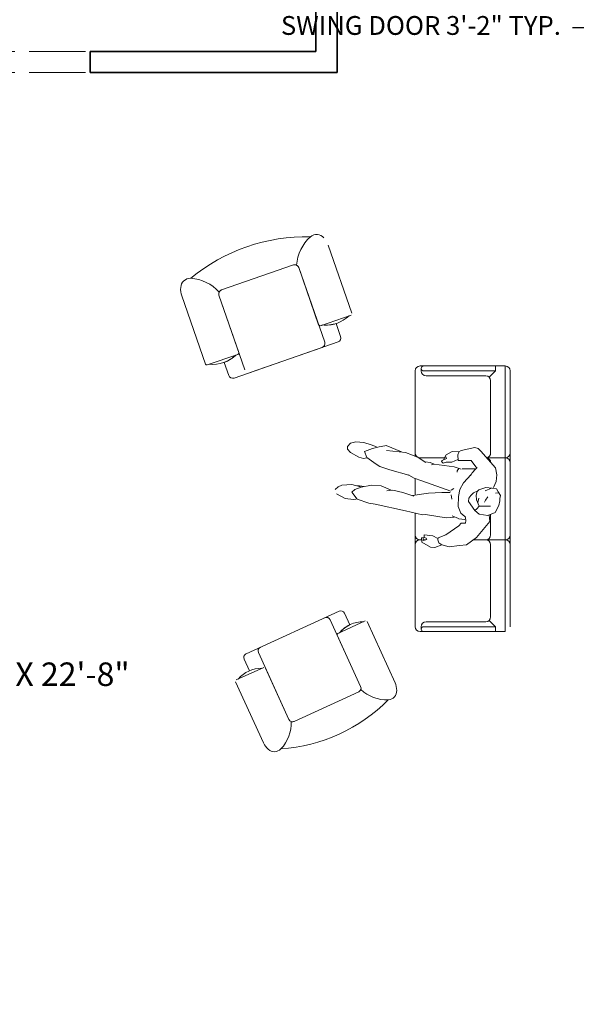
# Model space of a CAD drawing. Units: inches. Extents: x -638 to 186, y -762 to 59.
# Tile 14 of 31: x -287 to -168, y -413 to -203. Entities that reach past the tile are written whole.
import ezdxf

# ---------------------------------------------------------------- set-up
doc = ezdxf.new("R2010")
doc.units = ezdxf.units.IN
doc.linetypes.add('ACAD_ISO02W100', pattern=[15, 12, -3])
for name, color, linetype, lineweight in [('A-ANNO-DIMS', 2, 'Continuous', 18), ('A-AREA-IDEN', 1, 'Continuous', 18), ('A-ENTG-PEPL', 251, 'Continuous', 9), ('A-WALL-OVHD', 1, 'ACAD_ISO02W100', 18), ('furn', 8, 'Continuous', 13), ('wall', 7, 'Continuous', 35)]:
    doc.layers.add(name, color=color, linetype=linetype, lineweight=lineweight)
doc.styles.get("Standard").update_dxf_attribs({"font": 'arial.ttf'})
doc.dimstyles.new('ISO-25', dxfattribs={"dimtxt": 4, "dimasz": 4, "dimexe": 1.25, "dimexo": 0.625, "dimtad": 0, "dimlunit": 4, "dimtxsty": 'Standard', "dimcen": 2.5, "dimclrt": 256, "dimadec": 0, "dimazin": 0, "dimtfac": 1, "dimtmove": 0, "dimatfit": 3, "dimfxl": 1, "dimfxlon": 1, "dimarcsym": 0})

# ---------------------------------------------------------------- blocks, each defined once
blk = doc.blocks.new('*D23')
at = {"layer": 'A-ANNO-DIMS', "color": 0, "lineweight": -2, "transparency": 16777216}
for p, q in [((-165.01, -205.03), (-169.01, -205.03)), ((-165.01, -204.03), (-165.01, -206.28)), ((-131.22, -205.03), (-161.01, -205.03)), ((-127.22, -204.03), (-127.22, -206.28))]:
    blk.add_line(p, q, dxfattribs=at)
at = {"layer": 'A-ANNO-DIMS', "color": 0, "lineweight": 30, "transparency": 16777216}
for points in [[(-161.01, -204.37), (-161.01, -205.7), (-165.01, -205.03)], [(-131.22, -204.37), (-131.22, -205.7), (-127.22, -205.03)]]:
    blk.add_solid(points, dxfattribs=at)
at = {"layer": 'Defpoints', "color": 0, "lineweight": 30, "transparency": 16777216}
for p in [(-165.01, -199.36), (-127.22, -199.36), (-165.01, -205.03)]:
    blk.add_point(p, dxfattribs=at)
at = {"layer": 'A-ANNO-DIMS', "transparency": 16777216, "insert": (-201.22, -205.03), "char_height": 4, "attachment_point": 5}
blk.add_mtext('SWING DOOR 3\'-2" TYP.', dxfattribs=at)
blk = doc.blocks.new('*D37')
at = {"layer": 'A-ANNO-DIMS', "color": 0, "lineweight": -2, "transparency": 16777216}
for p, q in [((182.66, -232.53), (184.91, -232.53)), ((183.66, -236.53), (183.66, -250.51)), ((183.66, -276.53), (183.66, -262.56)), ((182.66, -280.53), (184.91, -280.53))]:
    blk.add_line(p, q, dxfattribs=at)
at = {"layer": 'A-ANNO-DIMS', "color": 0, "lineweight": 30, "transparency": 16777216}
for points in [[(183, -236.53), (184.33, -236.53), (183.66, -232.53)], [(183, -276.53), (184.33, -276.53), (183.66, -280.53)]]:
    blk.add_solid(points, dxfattribs=at)
at = {"layer": 'Defpoints', "color": 0, "lineweight": 30, "transparency": 16777216}
for p in [(-404.53, -232.53), (-404.53, -280.53), (183.66, -280.53)]:
    blk.add_point(p, dxfattribs=at)
at = {"layer": 'A-ANNO-DIMS', "transparency": 16777216, "insert": (183.66, -256.53), "char_height": 4, "attachment_point": 5, "rotation": 90}
blk.add_mtext('4\'-0"', dxfattribs=at)
blk = doc.blocks.new('*D38')
at = {"layer": 'A-ANNO-DIMS', "color": 0, "lineweight": -2, "transparency": 16777216}
for p, q in [((182.66, -280.53), (184.91, -280.53)), ((183.66, -284.53), (183.66, -371.73)), ((183.66, -473.53), (183.66, -386.34)), ((182.66, -477.53), (184.91, -477.53))]:
    blk.add_line(p, q, dxfattribs=at)
at = {"layer": 'A-ANNO-DIMS', "color": 0, "lineweight": 30, "transparency": 16777216}
for points in [[(183, -284.53), (184.33, -284.53), (183.66, -280.53)], [(183, -473.53), (184.33, -473.53), (183.66, -477.53)]]:
    blk.add_solid(points, dxfattribs=at)
at = {"layer": 'Defpoints', "color": 0, "lineweight": 30, "transparency": 16777216}
for p in [(-404.53, -280.53), (-404.53, -477.53), (183.66, -477.53)]:
    blk.add_point(p, dxfattribs=at)
at = {"layer": 'A-ANNO-DIMS', "transparency": 16777216, "insert": (183.66, -379.03), "char_height": 4, "attachment_point": 5, "rotation": 90}
blk.add_mtext('16\'-5"', dxfattribs=at)
blk = doc.blocks.new('*D39')
at = {"layer": 'A-ANNO-DIMS', "color": 0, "lineweight": -2, "transparency": 16777216}
for p, q in [((-344.53, -751.58), (-344.53, -753.83)), ((-340.53, -752.58), (-313.98, -752.58)), ((-275.53, -752.58), (-302.07, -752.58)), ((-271.53, -751.58), (-271.53, -753.83))]:
    blk.add_line(p, q, dxfattribs=at)
at = {"layer": 'A-ANNO-DIMS', "color": 0, "lineweight": 30, "transparency": 16777216}
for points in [[(-340.53, -751.92), (-340.53, -753.25), (-344.53, -752.58)], [(-275.53, -751.92), (-275.53, -753.25), (-271.53, -752.58)]]:
    blk.add_solid(points, dxfattribs=at)
at = {"layer": 'Defpoints', "color": 0, "lineweight": 30, "transparency": 16777216}
for p in [(-344.53, -214.53), (-271.53, -214.53), (-271.53, -752.58)]:
    blk.add_point(p, dxfattribs=at)
at = {"layer": 'A-ANNO-DIMS', "transparency": 16777216, "insert": (-308.03, -752.58), "char_height": 4, "attachment_point": 5}
blk.add_mtext('6\'-1"', dxfattribs=at)

msp = doc.modelspace()

# ---------------------------------------------------------------- linework, layer by layer
at = {"layer": 'A-ENTG-PEPL'}
for p, q in [((-216.835, -293.995, -103.961), (-216.211, -293.311, -103.961)), ((-216.815, -294.538, -103.961), (-216.835, -293.995, -103.961)), ((-216.177, -295.242, -103.961), (-216.815, -294.538, -103.961)), ((-216.211, -293.311, -103.961), (-215.063, -292.962, -103.961)), ((-215.063, -292.962, -103.961), (-213.387, -293.116, -103.961)), ((-213.387, -293.116, -103.961), (-211.817, -293.608, -103.961)), ((-213.188, -295.08, -103.961), (-211.493, -294.43, -103.961)), ((-211.817, -293.608, -103.961), (-210.649, -294.059, -103.961)), ((-211.493, -294.43, -103.961), (-210.106, -294.039, -103.961)), ((-210.106, -294.039, -103.961), (-208.904, -293.867, -103.961)), ((-208.904, -293.867, -103.961), (-208.573, -293.753, -103.961)), ((-208.573, -293.753, -103.961), (-205.378, -295.108, -103.961)), ((-208.52, -294.842, -103.961), (-204.514, -295.28, -103.961)), ((-195.875, -295.771), (-194.564, -295.027)), ((-194.564, -295.027), (-193.121, -295.142)), ((-193.121, -295.142), (-192.669, -294.855)), ((-192.669, -294.855), (-189.735, -294.232)), ((-189.735, -294.232), (-189.03, -294.413)), ((-189.03, -294.413), (-188.458, -294.991)), ((-188.458, -294.991), (-185.351, -298.556, -103.961)), ((-214.414, -296.274, -103.961), (-216.177, -295.242, -103.961)), ((-213.436, -296.52, -103.961), (-214.414, -296.274, -103.961)), ((-212.735, -296.388, -103.961), (-213.436, -296.52, -103.961)), ((-212.688, -296.316, -103.961), (-213.188, -295.08, -103.961)), ((-210.712, -297.729, -103.961), (-212.688, -296.316, -103.961)), ((-204.514, -295.28, -103.961), (-202.973, -295.856, -103.961)), ((-202.973, -295.856, -103.961), (-201.815, -296.356, -103.961)), ((-201.815, -296.356, -103.961), (-200.175, -297.401, -103.961)), ((-196.67, -296.982), (-196.806, -297.191)), ((-196.67, -296.982), (-195.765, -296.518)), ((-196.32, -296.676), (-195.875, -295.771)), ((-195.765, -296.518), (-195.896, -296.159)), ((-193.355, -296.756), (-194.665, -297.298)), ((-193.127, -295.196), (-193.37, -295.735)), ((-193.37, -295.735), (-193.317, -296.948)), ((-193.317, -296.948), (-190.55, -296.991)), ((-190.55, -296.991), (-189.32, -298.565, -103.961)), ((-209.917, -298.247, -103.961), (-210.712, -297.729, -103.961)), ((-207.845, -298.929, -103.961), (-209.917, -298.247, -103.961)), ((-203.782, -300.115, -103.961), (-207.845, -298.929, -103.961)), ((-200.331, -297.281, -103.961), (-199.269, -297.364, -103.961)), ((-199.269, -297.364, -103.961), (-198.397, -297.755, -103.961)), ((-198.931, -297.919, -103.961), (-198.39, -297.718, -103.961)), ((-198.39, -297.718, -103.961), (-194.161, -298.329, -103.961)), ((-196.513, -297.53), (-196.806, -297.191)), ((-195.867, -297.33), (-196.513, -297.53)), ((-194.665, -297.298), (-195.867, -297.33)), ((-194.161, -298.329, -103.961), (-192.64, -298.812, -103.961)), ((-193.188, -298.664, -103.961), (-193.508, -299.125, -103.961)), ((-193.508, -299.125, -103.961), (-193.486, -299.452, -103.961)), ((-192.45, -298.76, -103.961), (-191.409, -298.749, -103.961)), ((-191.409, -298.749, -103.961), (-189.755, -298.757, -103.961)), ((-189.629, -298.834, -103.961), (-190.319, -299.594, -103.961)), ((-189.226, -298.484, -103.961), (-189.629, -298.834, -103.961)), ((-185.351, -298.556, -103.961), (-185.049, -299.992, -103.961)), ((-203.782, -300.115, -103.961), (-203.821, -299.978, -103.961)), ((-202.685, -300.726, -103.961), (-203.782, -300.115, -103.961)), ((-200.998, -301.28, -103.961), (-202.685, -300.726, -103.961)), ((-194.89, -303.475, -103.961), (-200.998, -301.28, -103.961)), ((-190.524, -299.913, -103.961), (-192.137, -301.697, -103.961)), ((-190.319, -299.594, -103.961), (-190.679, -300.242, -103.961)), ((-185.049, -299.992, -103.961), (-185.211, -301.458, -103.961)), ((-219.423, -303.098, -103.961), (-218.814, -302.584, -103.961)), ((-218.814, -302.584, -103.961), (-218.02, -302.204, -103.961)), ((-218.02, -302.204, -103.961), (-215.922, -302.044, -103.961)), ((-215.922, -302.044, -103.961), (-214.027, -302.563, -103.961)), ((-215.893, -303.705, -103.961), (-215.286, -303.107, -103.961)), ((-215.286, -303.107, -103.961), (-213.932, -302.62, -103.961)), ((-214.668, -302.298, -103.961), (-213.373, -302.519, -103.961)), ((-213.932, -302.62, -103.961), (-211.693, -302.205, -103.961)), ((-211.693, -302.205, -103.961), (-209.641, -302.372, -103.961)), ((-209.641, -302.372, -103.961), (-207.54, -303.263, -103.961)), ((-208.489, -303.396, -103.961), (-207.152, -303.296, -103.961)), ((-207.152, -303.296, -103.961), (-205.035, -303.762, -103.961)), ((-194.786, -303.274, -103.961), (-194.204, -302.912, -103.961)), ((-192.965, -303.149, -103.961), (-193.25, -304.581, -103.961)), ((-192.137, -301.697, -103.961), (-192.965, -303.149, -103.961)), ((-189.126, -303.386, -103.961), (-190.044, -303.82, -103.961)), ((-188.931, -303.195, -103.961), (-189.227, -303.585, -103.961)), ((-187.394, -302.692, -103.961), (-188.931, -303.195, -103.961)), ((-187.557, -303.377, -103.961), (-186.242, -302.844, -103.961)), ((-186.071, -302.814, -103.961), (-187.394, -302.692, -103.961)), ((-185.15, -302.959, -103.961), (-186.071, -302.814, -103.961)), ((-185.211, -301.458, -103.961), (-185.814, -302.686, -103.961)), ((-184.801, -303.657, -103.961), (-185.15, -302.959, -103.961)), ((-217.289, -305.044, -103.961), (-219.156, -304.044, -103.961)), ((-215.536, -305.265, -103.961), (-217.289, -305.044, -103.961)), ((-214.78, -305.19, -103.961), (-215.893, -303.705, -103.961)), ((-215.07, -305.178, -103.961), (-215.536, -305.265, -103.961)), ((-212.314, -306.034, -103.961), (-214.78, -305.19, -103.961)), ((-205.035, -303.762, -103.961), (-202.744, -304.521, -103.961)), ((-202.994, -304.404, -103.961), (-199.629, -303.94, -103.961)), ((-199.629, -303.94, -103.961), (-196.765, -303.74, -103.961)), ((-196.765, -303.74, -103.961), (-194.968, -303.738, -103.961)), ((-194.631, -305.204, -103.961), (-194.805, -304.271, -103.961)), ((-193.25, -304.581, -103.961), (-193.275, -306.77, -103.961)), ((-190.993, -304.979, -103.961), (-191.08, -305.71, -103.961)), ((-190.606, -304.388, -103.961), (-190.993, -304.979, -103.961)), ((-190.044, -303.82, -103.961), (-190.606, -304.388, -103.961)), ((-189.227, -303.585, -103.961), (-189.468, -304.345, -103.961)), ((-189.468, -304.345, -103.961), (-189.398, -305.347, -103.961)), ((-189.398, -305.347, -103.961), (-188.815, -306.67, -103.961)), ((-188.92, -304.942, -103.961), (-189.136, -305.883, -103.961)), ((-187.478, -305.37, -103.961), (-187.725, -305.823, -103.961)), ((-186.993, -304.697, -103.961), (-187.478, -305.37, -103.961)), ((-184.78, -303.802, -103.961), (-185.339, -303.91, -103.961)), ((-184.317, -304.383, -103.961), (-184.801, -303.657, -103.961)), ((-184.454, -305.044, -103.961), (-184.317, -304.383, -103.961)), ((-184.412, -305.57, -103.961), (-184.454, -305.044, -103.961)), ((-210.974, -306.263, -103.961), (-212.314, -306.034, -103.961)), ((-204.51, -307.639, -103.961), (-210.974, -306.263, -103.961)), ((-193.275, -306.77, -103.961), (-192.748, -308.184, -103.961)), ((-191.08, -305.71, -103.961), (-189.719, -307.557, -103.961)), ((-189.335, -307.229, -103.961), (-189.719, -307.557, -103.961)), ((-189.719, -307.557, -103.961), (-188.833, -308.373, -103.961)), ((-188.815, -306.67, -103.961), (-189.335, -307.229, -103.961)), ((-188.789, -306.694, -103.961), (-186.434, -306.685, -103.961)), ((-185.439, -308.022, -103.961), (-184.66, -306.56, -103.961)), ((-184.66, -306.56, -103.961), (-184.412, -305.57, -103.961)), ((-200.893, -308.488, -103.961), (-204.51, -307.639, -103.961)), ((-200.254, -308.435, -103.961), (-200.893, -308.488, -103.961)), ((-195.813, -309.14, -103.961), (-200.254, -308.435, -103.961)), ((-194.151, -308.971, -103.961), (-195.813, -309.14, -103.961)), ((-193.238, -309.293, -103.961), (-194.562, -308.721, -103.961)), ((-191.848, -309.531, -103.961), (-193.162, -309.359, -103.961)), ((-192.748, -308.184, -103.961), (-191.901, -308.892, -103.961)), ((-191.787, -308.773, -103.961), (-191.663, -309.696, -103.961)), ((-188.833, -308.373, -103.961), (-186.964, -308.655, -103.961)), ((-186.964, -308.655, -103.961), (-185.439, -308.022, -103.961)), ((-186.593, -309.949, -103.961), (-186.67, -308.534, -103.961)), ((-193.152, -310.851, -103.961), (-195.932, -312.79, -103.961)), ((-192.639, -310.301, -103.961), (-193.152, -310.851, -103.961)), ((-191.71, -310.275, -103.961), (-192.639, -310.301, -103.961)), ((-191.663, -309.696, -103.961), (-191.71, -310.275, -103.961)), ((-189.365, -313.299, -103.961), (-186.593, -309.949, -103.961)), ((-199.973, -313.761, -103.961), (-200.745, -313.967, -103.961)), ((-200.503, -312.769, -103.961), (-200.56, -313.334, -103.961)), ((-200.56, -313.334, -103.961), (-200.123, -313.481, -103.961)), ((-198.655, -312.994, -103.961), (-200.503, -312.769, -103.961)), ((-200.123, -313.481, -103.961), (-199.973, -313.761, -103.961)), ((-197.618, -313.546, -103.961), (-198.655, -312.994, -103.961)), ((-197.647, -313.801, -103.961), (-197.579, -313.371, -103.961)), ((-197.41, -314.432, -103.961), (-197.647, -313.801, -103.961)), ((-195.932, -312.79, -103.961), (-197.579, -313.371, -103.961)), ((-191.503, -314.852, -103.961), (-189.365, -313.299, -103.961)), ((-199.185, -315.357, -103.961), (-198.267, -315.446, -103.961)), ((-198.267, -315.446, -103.961), (-196.79, -314.918, -103.961)), ((-196.79, -314.918, -103.961), (-197.41, -314.432, -103.961)), ((-196.79, -314.918, -103.961), (-195.242, -315.29, -103.961)), ((-195.242, -315.29, -103.961), (-193.029, -315.062, -103.961)), ((-193.029, -315.062, -103.961), (-191.503, -314.852, -103.961))]:
    msp.add_line(p, q, dxfattribs=at)
at = {"layer": 'A-ENTG-PEPL', "elevation": -103.961}
msp.add_lwpolyline([(-200.745, -313.967), (-200.703, -313.293), (-201.105, -313.383), (-201.046, -314.329), (-199.185, -315.357)], dxfattribs=at)
at = {"layer": 'A-WALL-OVHD'}
for p, q in [((-344.526, -210.033), (-271.526, -210.033)), ((-344.526, -214.533), (-271.526, -214.533))]:
    msp.add_line(p, q, dxfattribs=at)
at = {"layer": 'furn'}
for p, q in [((-215.879, -265.669), (-220.912, -251.167)), ((-243.612, -260.703), (-228.325, -255.398)), ((-228.325, -255.398), (-243.612, -260.703)), ((-228.325, -255.398), (-243.612, -260.703)), ((-227.181, -255.952), (-222.956, -268.125)), ((-227.181, -255.952), (-222.956, -268.125)), ((-221.679, -271.806), (-227.181, -255.952)), ((-247.019, -276.476), (-252.052, -261.974)), ((-239.942, -274.02), (-244.166, -261.847)), ((-244.166, -261.847), (-238.665, -277.7)), ((-244.166, -261.847), (-239.942, -274.02)), ((-222.575, -268.31), (-216.064, -266.051)), ((-222.575, -268.31), (-222.15, -268.163)), ((-219.242, -267.861), (-218.282, -270.627)), ((-218.836, -271.771), (-240.918, -279.434)), ((-237.521, -278.255), (-222.234, -272.95)), ((-240.127, -274.401), (-246.638, -276.661)), ((-242.062, -278.879), (-243.022, -276.114)), ((-240.551, -274.549), (-240.127, -274.401)), ((-202.44, -277.914), (-202.44, -296.086)), ((-200.642, -276.878), (-201.405, -276.878)), ((-201.16, -277.396), (-201.16, -277.914)), ((-200.642, -276.878), (-183.283, -276.878)), ((-185.354, -277.914), (-200.642, -277.914)), ((-186.693, -279.253), (-185.354, -277.914)), ((-185.354, -277.914), (-185.354, -276.878)), ((-182.247, -277.914), (-182.247, -332.28)), ((-200.124, -278.949), (-187.425, -278.949)), ((-186.389, -279.985), (-186.389, -295.345)), ((-196.175, -296.381), (-201.405, -296.381)), ((-183.283, -296.381), (-187.247, -296.381)), ((-202.44, -300.807), (-202.44, -304.328)), ((-202.44, -308.125), (-202.44, -332.28)), ((-186.389, -308.417), (-186.389, -312.777)), ((-201.078, -313.813), (-201.405, -313.813)), ((-200.168, -313.813), (-200.735, -313.813)), ((-183.283, -313.813), (-190.072, -313.813)), ((-186.389, -314.848), (-186.389, -330.209)), ((-218.594, -328.993), (-238.404, -338.051)), ((-216.35, -331.887), (-217.484, -329.406)), ((-220.532, -330.8), (-214.029, -345.022)), ((-218.884, -333.731), (-213.043, -331.06)), ((-212.673, -331.198), (-206.724, -344.209)), ((-201.16, -332.797), (-201.16, -332.28)), ((-185.354, -332.28), (-200.642, -332.28)), ((-187.425, -331.244), (-200.124, -331.244)), ((-186.693, -330.941), (-185.354, -332.28)), ((-185.354, -332.28), (-185.354, -333.315)), ((-214.029, -345.022), (-219.022, -334.101)), ((-214.029, -345.022), (-219.022, -334.101)), ((-218.884, -333.731), (-218.503, -333.557)), ((-200.642, -333.315), (-201.405, -333.315)), ((-183.283, -333.315), (-200.642, -333.315)), ((-229.267, -351.99), (-235.77, -337.767)), ((-234.63, -340.931), (-240.472, -343.602)), ((-238.818, -339.161), (-237.683, -341.642)), ((-229.267, -351.99), (-234.26, -341.069)), ((-234.26, -341.069), (-229.267, -351.99)), ((-240.61, -343.972), (-234.661, -356.983)), ((-214.442, -346.132), (-228.157, -352.403)), ((-214.442, -346.132), (-228.157, -352.403)), ((-228.157, -352.403), (-214.442, -346.132))]:
    msp.add_line(p, q, dxfattribs=at)
msp.add_lwpolyline([(-183.283, -276.878), (-183.283, -333.315)], dxfattribs=at)
for centre, radius, start, end in [((-223.381, -251.032), 2.098, 42.15096, 129.53897), ((-225.567, -288.022), 38.617, 88.73747, 129.53993), ((-218.732, -256.037), 8.926, 132.10071, 176.15197), ((-218.732, -256.037), 8.926, 132.10071, 176.15197), ((-228.03, -256.247), 0.899, 64.1387, 109.1387), ((-228.03, -256.247), 0.899, 19.1387, 109.1387), ((-228.03, -256.247), 0.899, 64.1387, 109.1387), ((-228.03, -256.247), 0.899, 19.1387, 64.1387), ((-228.03, -256.247), 0.899, 19.1387, 64.1387), ((-250.198, -260.338), 2.098, 88.73843, 176.12644), ((-250.747, -267.148), 8.926, 42.12543, 86.17668), ((-250.747, -267.148), 8.926, 42.12543, 86.17668), ((-247.806, -260.5), 4.495, 176.12644, 199.1387), ((-243.317, -261.552), 0.899, 109.1387, 199.1387), ((-243.317, -261.552), 0.899, 154.1387, 199.1387), ((-243.317, -261.552), 0.899, 154.1387, 199.1387), ((-243.317, -261.552), 0.899, 109.1387, 154.1387), ((-243.317, -261.552), 0.899, 109.1387, 154.1387), ((-221.406, -261.166), 7.036, 263.93143, 314.34596), ((-222.673, -268.027), 0.3, 199.1387, 289.1387), ((-222.673, -268.027), 0.3, 199.1387, 289.1387), ((-221.406, -261.166), 7.036, 263.93143, 287.91851), ((-222.528, -272.1), 0.899, 289.1387, 19.1387), ((-219.131, -270.921), 0.899, 289.1387, 19.1387), ((-240.225, -274.118), 0.3, 289.1387, 19.1387), ((-240.225, -274.118), 0.3, 289.1387, 19.1387), ((-245.469, -269.517), 7.036, 263.93143, 314.34596), ((-245.469, -269.517), 7.036, 290.35889, 314.34596), ((-246.736, -276.378), 0.3, 199.1387, 289.1387), ((-201.405, -277.914), 1.036, 90, 180), ((-200.642, -277.396), 0.518, 90, 270), ((-200.124, -277.914), 1.036, 180, 270), ((-183.283, -277.914), 1.036, 0, 90), ((-241.213, -278.584), 0.899, 199.1387, 289.1387), ((-187.425, -279.985), 1.036, 0, 90), ((-201.405, -295.345), 1.036, 180, 270), ((-201.405, -297.417), 1.036, 90, 106.92048), ((-187.425, -295.345), 1.036, 279.2298, 0), ((-187.425, -297.417), 1.036, 0, 79.2183), ((-183.283, -295.345), 1.036, 270, 0), ((-183.283, -297.417), 1.036, 0, 90), ((-201.405, -312.777), 1.036, 180, 270), ((-201.405, -314.848), 1.036, 90, 180), ((-187.425, -312.777), 1.036, 270, 0), ((-187.425, -314.848), 1.036, 0, 90), ((-183.283, -312.777), 1.036, 270, 0), ((-183.283, -314.848), 1.036, 0, 90), ((-221.294, -331.148), 0.838, 24.57225, 114.57225), ((-218.246, -329.755), 0.838, 24.57225, 114.57225), ((-187.425, -330.209), 1.036, 270, 0), ((-213.497, -337.791), 6.557, 89.36499, 139.77951), ((-213.497, -337.791), 6.557, 115.79244, 139.77951), ((-201.405, -332.28), 1.036, 180, 270), ((-200.124, -332.28), 1.036, 90, 180), ((-200.642, -332.797), 0.518, 90, 270), ((-218.768, -333.985), 0.279, 114.57225, 204.57225), ((-218.768, -333.985), 0.279, 114.57225, 204.57225), ((-235.008, -337.419), 0.838, 114.57225, 204.57225), ((-238.056, -338.813), 0.838, 114.57225, 204.57225), ((-235.084, -347.662), 6.557, 89.36499, 139.77951), ((-214.79, -345.371), 0.838, 294.57225, 24.57225), ((-214.79, -345.371), 0.838, 339.57225, 24.57225), ((-214.79, -345.371), 0.838, 339.57225, 24.57225), ((-210.533, -345.951), 4.189, 1.55999, 24.57225), ((-214.79, -345.371), 0.838, 294.57225, 339.57225), ((-214.79, -345.371), 0.838, 294.57225, 339.57225), ((-208.392, -339.524), 8.319, 227.55898, 271.61023), ((-208.392, -339.524), 8.319, 227.55898, 271.61023), ((-208.3, -345.89), 1.955, 274.17198, 1.55999), ((-233.594, -322.38), 35.989, 274.17102, 314.97348), ((-237.113, -352.657), 8.319, 317.53427, 1.58552), ((-237.113, -352.657), 8.319, 317.53427, 1.58552), ((-228.505, -351.641), 0.838, 204.57225, 294.57225), ((-228.505, -351.641), 0.838, 204.57225, 249.57225), ((-228.505, -351.641), 0.838, 204.57225, 249.57225), ((-228.505, -351.641), 0.838, 249.57225, 294.57225), ((-228.505, -351.641), 0.838, 249.57225, 294.57225), ((-230.851, -355.241), 4.189, 204.57225, 227.58451), ((-232.358, -356.89), 1.955, 227.58451, 314.97252)]:
    msp.add_arc(centre, radius, start, end, dxfattribs=at)
at = {"layer": 'wall'}
for p, q in [((-223.526, -210.033), (-223.526, -97.533)), ((-219.026, -214.533), (-219.026, -153.025)), ((-271.526, -214.533), (-271.526, -210.033)), ((-271.526, -210.033), (-223.526, -210.033)), ((-271.526, -214.533), (-223.526, -214.533)), ((-223.526, -214.533), (-219.026, -214.533))]:
    msp.add_line(p, q, dxfattribs=at)

# ---------------------------------------------------------------- texts
at = {"layer": 'A-AREA-IDEN', "insert": (-315.786, -329.852), "char_height": 5, "attachment_point": 1}
msp.add_mtext_dynamic_manual_height_columns('\\A1;LIVING\\P19\'-11 {\\H0.7x;\\S1/2;}" X 22\'-8"', width=96.10133, gutter_width=12.5, heights=[0], dxfattribs=at)

# ---------------------------------------------------------------- dimensions: what is measured, and where the dimension line sits
at = {"layer": 'A-ANNO-DIMS'}
dim = msp.add_linear_dim(base=(-165.015, -205.032), p1=(-127.219, -199.363), p2=(-165.015, -199.363), angle=180, text='SWING DOOR <> TYP.', dimstyle='ISO-25', override={"dimdec": 1, "dimlfac": 1, "dimrnd": 0, "dimzin": 1, "dimdsep": 46, "dimlunit": 4, "dimfrac": 2}, dxfattribs=at)
dim.commit()
dim.dimension.update_dxf_attribs({"geometry": '*D23', "text_midpoint": (-201.224, -205.032)})
dim = msp.add_linear_dim(base=(-271.526, -752.583), p1=(-344.526, -214.533), p2=(-271.526, -214.533), dimstyle='ISO-25', override={"dimdec": 1, "dimlfac": 1, "dimrnd": 0, "dimzin": 1, "dimdsep": 46, "dimlunit": 4, "dimfrac": 2}, dxfattribs=at)
dim.commit()
dim.dimension.update_dxf_attribs({"geometry": '*D39', "text_midpoint": (-308.026, -752.583)})
for base, p1, p2, picture, middle in [((183.663, -280.533), (-404.526, -232.533), (-404.526, -280.533), '*D37', (183.663, -256.533)), ((183.663, -477.533), (-404.526, -280.533), (-404.526, -477.533), '*D38', (183.663, -379.033))]:
    dim = msp.add_linear_dim(base=base, p1=p1, p2=p2, angle=90, dimstyle='ISO-25', override={"dimdec": 1, "dimlfac": 1, "dimrnd": 0, "dimzin": 1, "dimdsep": 46, "dimlunit": 4, "dimfrac": 2}, dxfattribs=at)
    dim.commit()
    dim.dimension.update_dxf_attribs({"geometry": picture, "text_midpoint": middle})

doc.saveas('drawing.dxf')
